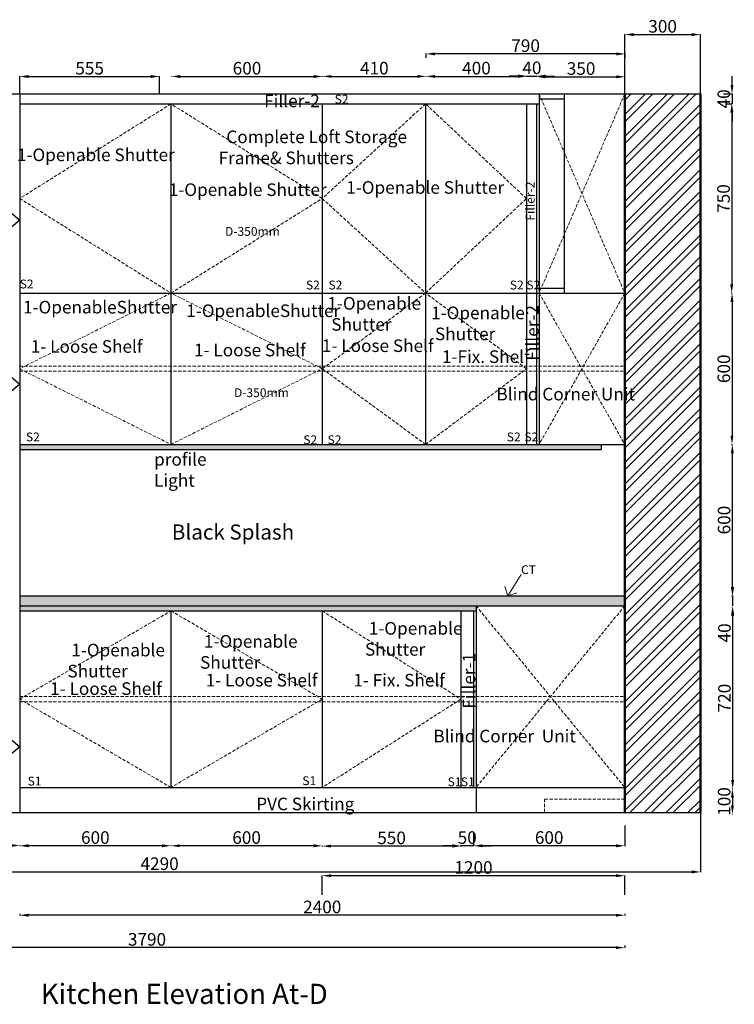
# Model space of a CAD drawing. Units: millimetres. Extents: x 407065 to 421840, y 1168257 to 1177792.
# Tile 14 of 17: x 415751 to 418585, y 1168277 to 1172181. Entities that reach past the tile are written whole.
import ezdxf

# ---------------------------------------------------------------- set-up
doc = ezdxf.new("R2010")
doc.units = ezdxf.units.MM
doc.linetypes.add('DASHED', pattern=[19.05, 12.7, -6.35])
for name, color, linetype, lineweight in [('A-ANNO-DIMS', 6, 'Continuous', 18), ('A-ANNO-SYMB', 6, 'Continuous', 18), ('A-ANNO-TEXT', 30, 'Continuous', 18), ('A-FURN', 3, 'Continuous', 25), ('A-FURN-HIDN', 7, 'DASHED', 18), ('A-FURN-PATT', 252, 'Continuous', 13), ('A-WALL', 7, 'Continuous', 50), ('A-WALL-PATT', 8, 'Continuous', 13)]:
    doc.layers.add(name, color=color, linetype=linetype, lineweight=lineweight)
doc.styles.get("Standard").update_dxf_attribs({"font": 'arial.ttf'})
doc.dimstyles.new('ISO-25', dxfattribs={"dimtxt": 50, "dimasz": 35, "dimexe": 1.25, "dimexo": 0.625, "dimtad": 1, "dimdec": 1, "dimtxsty": 'Standard', "dimcen": 35, "dimadec": 0, "dimazin": 0, "dimtfac": 1, "dimtdec": 1, "dimtmove": 0, "dimatfit": 3, "dimfxl": 1, "dimarcsym": 0})

# ---------------------------------------------------------------- blocks, each defined once
blk = doc.blocks.new('*D135')
at = {"layer": 'A-ANNO-DIMS', "color": 0, "lineweight": -2, "transparency": 16777216}
for p, q in [((415750.9, 1171887.4), (415750.9, 1171956.9)), ((415785.9, 1171955.6), (416270.9, 1171955.6)), ((416305.9, 1171887.4), (416305.9, 1171956.9))]:
    blk.add_line(p, q, dxfattribs=at)
at = {"layer": 'A-ANNO-DIMS', "color": 0, "transparency": 16777216}
for points in [[(415785.9, 1171961.5), (415785.9, 1171949.8), (415750.9, 1171955.6)], [(416270.9, 1171961.5), (416270.9, 1171949.8), (416305.9, 1171955.6)]]:
    blk.add_solid(points, dxfattribs=at)
at = {"layer": 'Defpoints', "color": 0, "transparency": 16777216}
for p in [(416305.9, 1171955.6), (415750.9, 1171886.8), (416305.9, 1171886.8)]:
    blk.add_point(p, dxfattribs=at)
at = {"layer": 'A-ANNO-DIMS', "color": 0, "transparency": 16777216, "insert": (416028.4, 1171981.7), "char_height": 50, "attachment_point": 5}
blk.add_mtext('555', dxfattribs=at)
blk = doc.blocks.new('*D136')
at = {"layer": 'A-ANNO-DIMS', "color": 0, "lineweight": -2, "transparency": 16777216}
for p, q in [((416352.5, 1171955.3), (416352.5, 1171954.4)), ((416387.5, 1171955.6), (416917.5, 1171955.6)), ((416952.5, 1171955.3), (416952.5, 1171954.4))]:
    blk.add_line(p, q, dxfattribs=at)
at = {"layer": 'A-ANNO-DIMS', "color": 0, "transparency": 16777216}
for points in [[(416387.5, 1171961.5), (416387.5, 1171949.8), (416352.5, 1171955.6)], [(416917.5, 1171961.5), (416917.5, 1171949.8), (416952.5, 1171955.6)]]:
    blk.add_solid(points, dxfattribs=at)
at = {"layer": 'Defpoints', "color": 0, "transparency": 16777216}
for p in [(416352.5, 1171955.9), (416952.5, 1171955.9), (416952.5, 1171955.6)]:
    blk.add_point(p, dxfattribs=at)
at = {"layer": 'A-ANNO-DIMS', "color": 0, "transparency": 16777216, "insert": (416652.5, 1171981.8), "char_height": 50, "attachment_point": 5}
blk.add_mtext('600', dxfattribs=at)
blk = doc.blocks.new('*D137')
at = {"layer": 'A-ANNO-DIMS', "color": 0, "lineweight": -2, "transparency": 16777216}
for p, q in [((416952.5, 1171955), (416952.5, 1171957.2)), ((416987.5, 1171955.9), (417327.5, 1171955.9)), ((417362.5, 1171955), (417362.5, 1171957.2))]:
    blk.add_line(p, q, dxfattribs=at)
at = {"layer": 'A-ANNO-DIMS', "color": 0, "transparency": 16777216}
for points in [[(416987.5, 1171961.7), (416987.5, 1171950.1), (416952.5, 1171955.9)], [(417327.5, 1171961.7), (417327.5, 1171950.1), (417362.5, 1171955.9)]]:
    blk.add_solid(points, dxfattribs=at)
at = {"layer": 'Defpoints', "color": 0, "transparency": 16777216}
for p in [(416952.5, 1171954.4), (417362.5, 1171955.9), (417362.5, 1171954.4)]:
    blk.add_point(p, dxfattribs=at)
at = {"layer": 'A-ANNO-DIMS', "color": 0, "transparency": 16777216, "insert": (417157.5, 1171982.1), "char_height": 50, "attachment_point": 5}
blk.add_mtext('410', dxfattribs=at)
blk = doc.blocks.new('*D138')
at = {"layer": 'A-ANNO-DIMS', "color": 0, "lineweight": -2, "transparency": 16777216}
for p, q in [((417362.5, 1171955), (417362.5, 1171957.3)), ((417397.5, 1171956.1), (417727.5, 1171956.1)), ((417762.5, 1171955), (417762.5, 1171957.3))]:
    blk.add_line(p, q, dxfattribs=at)
at = {"layer": 'A-ANNO-DIMS', "color": 0, "transparency": 16777216}
for points in [[(417397.5, 1171961.9), (417397.5, 1171950.2), (417362.5, 1171956.1)], [(417727.5, 1171961.9), (417727.5, 1171950.2), (417762.5, 1171956.1)]]:
    blk.add_solid(points, dxfattribs=at)
at = {"layer": 'Defpoints', "color": 0, "transparency": 16777216}
for p in [(417362.5, 1171954.4), (417762.5, 1171956.1), (417762.5, 1171954.4)]:
    blk.add_point(p, dxfattribs=at)
at = {"layer": 'A-ANNO-DIMS', "color": 0, "transparency": 16777216, "insert": (417562.5, 1171982.2), "char_height": 50, "attachment_point": 5}
blk.add_mtext('400', dxfattribs=at)
blk = doc.blocks.new('*D139')
at = {"layer": 'A-ANNO-DIMS', "color": 0, "lineweight": -2, "transparency": 16777216}
for p, q in [((417727.5, 1171957.3), (417692.5, 1171957.3)), ((417762.5, 1171955), (417762.5, 1171958.6)), ((417762.5, 1171957.3), (417802.5, 1171957.3)), ((417802.5, 1171955), (417802.5, 1171958.6)), ((417837.5, 1171957.3), (417872.5, 1171957.3))]:
    blk.add_line(p, q, dxfattribs=at)
at = {"layer": 'A-ANNO-DIMS', "color": 0, "transparency": 16777216}
for points in [[(417727.5, 1171963.2), (417727.5, 1171951.5), (417762.5, 1171957.3)], [(417837.5, 1171963.2), (417837.5, 1171951.5), (417802.5, 1171957.3)]]:
    blk.add_solid(points, dxfattribs=at)
at = {"layer": 'Defpoints', "color": 0, "transparency": 16777216}
for p in [(417762.5, 1171954.4), (417802.5, 1171957.3), (417802.5, 1171954.4)]:
    blk.add_point(p, dxfattribs=at)
at = {"layer": 'A-ANNO-DIMS', "color": 0, "transparency": 16777216, "insert": (417782.5, 1171983.5), "char_height": 50, "attachment_point": 5}
blk.add_mtext('40', dxfattribs=at)
blk = doc.blocks.new('*D140')
at = {"layer": 'A-ANNO-DIMS', "color": 0, "lineweight": -2, "transparency": 16777216}
for p, q in [((417802.5, 1171955), (417802.5, 1171955.6)), ((417837.5, 1171954.4), (418117.5, 1171954.4)), ((418152.5, 1171955), (418152.5, 1171955.6))]:
    blk.add_line(p, q, dxfattribs=at)
at = {"layer": 'A-ANNO-DIMS', "color": 0, "transparency": 16777216}
for points in [[(417837.5, 1171960.2), (417837.5, 1171948.5), (417802.5, 1171954.4)], [(418117.5, 1171960.2), (418117.5, 1171948.5), (418152.5, 1171954.4)]]:
    blk.add_solid(points, dxfattribs=at)
at = {"layer": 'Defpoints', "color": 0, "transparency": 16777216}
for p in [(417802.5, 1171954.4), (418152.5, 1171954.4), (418152.5, 1171954.4)]:
    blk.add_point(p, dxfattribs=at)
at = {"layer": 'A-ANNO-DIMS', "color": 0, "transparency": 16777216, "insert": (417977.5, 1171980.6), "char_height": 50, "attachment_point": 5}
blk.add_mtext('350', dxfattribs=at)
blk = doc.blocks.new('*D141')
at = {"layer": 'A-ANNO-DIMS', "color": 0, "lineweight": -2, "transparency": 16777216}
for p, q in [((417362.5, 1172030), (417362.5, 1172046.4)), ((418117.5, 1172045.1), (417397.5, 1172045.1)), ((418152.5, 1172030), (418152.5, 1172046.4))]:
    blk.add_line(p, q, dxfattribs=at)
at = {"layer": 'A-ANNO-DIMS', "color": 0, "transparency": 16777216}
for points in [[(417397.5, 1172050.9), (417397.5, 1172039.3), (417362.5, 1172045.1)], [(418117.5, 1172050.9), (418117.5, 1172039.3), (418152.5, 1172045.1)]]:
    blk.add_solid(points, dxfattribs=at)
at = {"layer": 'Defpoints', "color": 0, "transparency": 16777216}
for p in [(417362.5, 1172045.1), (417362.5, 1172029.4), (418152.5, 1172029.4)]:
    blk.add_point(p, dxfattribs=at)
at = {"layer": 'A-ANNO-DIMS', "color": 0, "transparency": 16777216, "insert": (417757.5, 1172071.3), "char_height": 50, "attachment_point": 5}
blk.add_mtext('790', dxfattribs=at)
blk = doc.blocks.new('*D142')
at = {"layer": 'A-ANNO-DIMS', "color": 0, "lineweight": -2, "transparency": 16777216}
for p, q in [((418576.1, 1171921.8), (418576.1, 1171956.8)), ((418542.5, 1171886.8), (418577.4, 1171886.8)), ((418576.1, 1171886.8), (418576.1, 1171846.8)), ((418551.7, 1171846.8), (418577.4, 1171846.8)), ((418576.1, 1171811.8), (418576.1, 1171776.8))]:
    blk.add_line(p, q, dxfattribs=at)
at = {"layer": 'A-ANNO-DIMS', "color": 0, "transparency": 16777216}
for points in [[(418570.3, 1171921.8), (418581.9, 1171921.8), (418576.1, 1171886.8)], [(418570.3, 1171811.8), (418581.9, 1171811.8), (418576.1, 1171846.8)]]:
    blk.add_solid(points, dxfattribs=at)
at = {"layer": 'Defpoints', "color": 0, "transparency": 16777216}
for p in [(418541.8, 1171886.8), (418551, 1171846.8), (418576.1, 1171846.8)]:
    blk.add_point(p, dxfattribs=at)
at = {"layer": 'A-ANNO-DIMS', "color": 0, "transparency": 16777216, "insert": (418550, 1171866.8), "char_height": 50, "attachment_point": 5, "rotation": 90}
blk.add_mtext('40', dxfattribs=at)
blk = doc.blocks.new('*D143')
at = {"layer": 'A-ANNO-DIMS', "color": 0, "lineweight": -2, "transparency": 16777216}
for p, q in [((418575.5, 1171846.8), (418573.7, 1171846.8)), ((418574.9, 1171811.8), (418574.9, 1171131.8)), ((418575.5, 1171096.8), (418573.7, 1171096.8))]:
    blk.add_line(p, q, dxfattribs=at)
at = {"layer": 'A-ANNO-DIMS', "color": 0, "transparency": 16777216}
for points in [[(418569.1, 1171811.8), (418580.7, 1171811.8), (418574.9, 1171846.8)], [(418569.1, 1171131.8), (418580.7, 1171131.8), (418574.9, 1171096.8)]]:
    blk.add_solid(points, dxfattribs=at)
at = {"layer": 'Defpoints', "color": 0, "transparency": 16777216}
for p in [(418576.1, 1171846.8), (418574.9, 1171096.8), (418576.1, 1171096.8)]:
    blk.add_point(p, dxfattribs=at)
at = {"layer": 'A-ANNO-DIMS', "color": 0, "transparency": 16777216, "insert": (418548.8, 1171471.8), "char_height": 50, "attachment_point": 5, "rotation": 90}
blk.add_mtext('750', dxfattribs=at)
blk = doc.blocks.new('*D144')
at = {"layer": 'A-ANNO-DIMS', "color": 0, "lineweight": -2, "transparency": 16777216}
for p, q in [((418574.3, 1171096.8), (418577.4, 1171096.8)), ((418576.1, 1171061.8), (418576.1, 1170531.8)), ((418574.3, 1170496.8), (418577.4, 1170496.8))]:
    blk.add_line(p, q, dxfattribs=at)
at = {"layer": 'A-ANNO-DIMS', "color": 0, "transparency": 16777216}
for points in [[(418570.3, 1171061.8), (418581.9, 1171061.8), (418576.1, 1171096.8)], [(418570.3, 1170531.8), (418581.9, 1170531.8), (418576.1, 1170496.8)]]:
    blk.add_solid(points, dxfattribs=at)
at = {"layer": 'Defpoints', "color": 0, "transparency": 16777216}
for p in [(418573.7, 1171096.8), (418573.7, 1170496.8), (418576.1, 1170496.8)]:
    blk.add_point(p, dxfattribs=at)
at = {"layer": 'A-ANNO-DIMS', "color": 0, "transparency": 16777216, "insert": (418550, 1170796.8), "char_height": 50, "attachment_point": 5, "rotation": 90}
blk.add_mtext('600', dxfattribs=at)
blk = doc.blocks.new('*D145')
at = {"layer": 'A-ANNO-DIMS', "color": 0, "lineweight": -2, "transparency": 16777216}
for p, q in [((418574.3, 1170496.8), (418578.6, 1170496.8)), ((418577.4, 1170461.8), (418577.4, 1169931.8)), ((418574.3, 1169896.8), (418578.6, 1169896.8))]:
    blk.add_line(p, q, dxfattribs=at)
at = {"layer": 'A-ANNO-DIMS', "color": 0, "transparency": 16777216}
for points in [[(418571.5, 1170461.8), (418583.2, 1170461.8), (418577.4, 1170496.8)], [(418571.5, 1169931.8), (418583.2, 1169931.8), (418577.4, 1169896.8)]]:
    blk.add_solid(points, dxfattribs=at)
at = {"layer": 'Defpoints', "color": 0, "transparency": 16777216}
for p in [(418573.7, 1170496.8), (418573.7, 1169896.8), (418577.4, 1169896.8)]:
    blk.add_point(p, dxfattribs=at)
at = {"layer": 'A-ANNO-DIMS', "color": 0, "transparency": 16777216, "insert": (418551.2, 1170196.8), "char_height": 50, "attachment_point": 5, "rotation": 90}
blk.add_mtext('600', dxfattribs=at)
blk = doc.blocks.new('*D146')
at = {"layer": 'A-ANNO-DIMS', "color": 0, "lineweight": -2, "transparency": 16777216}
for p, q in [((418578.6, 1169931.8), (418578.6, 1169966.8)), ((418578.6, 1169896.8), (418578.6, 1169856.8)), ((418579.2, 1169896.8), (418579.9, 1169896.8)), ((418579.2, 1169856.8), (418579.9, 1169856.8)), ((418578.6, 1169821.8), (418578.6, 1169712.1))]:
    blk.add_line(p, q, dxfattribs=at)
at = {"layer": 'A-ANNO-DIMS', "color": 0, "transparency": 16777216}
for points in [[(418572.8, 1169931.8), (418584.4, 1169931.8), (418578.6, 1169896.8)], [(418572.8, 1169821.8), (418584.4, 1169821.8), (418578.6, 1169856.8)]]:
    blk.add_solid(points, dxfattribs=at)
at = {"layer": 'Defpoints', "color": 0, "transparency": 16777216}
for p in [(418578.6, 1169896.8), (418578.6, 1169856.8), (418578.6, 1169856.8)]:
    blk.add_point(p, dxfattribs=at)
at = {"layer": 'A-ANNO-DIMS', "color": 0, "transparency": 16777216, "insert": (418552.5, 1169749.5), "char_height": 50, "attachment_point": 5, "rotation": 90}
blk.add_mtext('40', dxfattribs=at)
blk = doc.blocks.new('*D147')
at = {"layer": 'A-ANNO-DIMS', "color": 0, "lineweight": -2, "transparency": 16777216}
for p, q in [((418579.2, 1169851.1), (418579.9, 1169851.1)), ((418578.6, 1169816.1), (418578.6, 1169166.1)), ((418579.2, 1169131.1), (418579.9, 1169131.1))]:
    blk.add_line(p, q, dxfattribs=at)
at = {"layer": 'A-ANNO-DIMS', "color": 0, "transparency": 16777216}
for points in [[(418572.8, 1169816.1), (418584.4, 1169816.1), (418578.6, 1169851.1)], [(418572.8, 1169166.1), (418584.4, 1169166.1), (418578.6, 1169131.1)]]:
    blk.add_solid(points, dxfattribs=at)
at = {"layer": 'Defpoints', "color": 0, "transparency": 16777216}
for p in [(418578.6, 1169851.1), (418578.6, 1169131.1), (418578.6, 1169131.1)]:
    blk.add_point(p, dxfattribs=at)
at = {"layer": 'A-ANNO-DIMS', "color": 0, "transparency": 16777216, "insert": (418552.5, 1169491.1), "char_height": 50, "attachment_point": 5, "rotation": 90}
blk.add_mtext('720', dxfattribs=at)
blk = doc.blocks.new('*D148')
at = {"layer": 'A-ANNO-DIMS', "color": 0, "lineweight": -2, "transparency": 16777216}
for p, q in [((418578, 1169131.1), (418576.4, 1169131.1)), ((418577.7, 1169096.1), (418577.7, 1169066.1)), ((418578, 1169031.1), (418576.4, 1169031.1))]:
    blk.add_line(p, q, dxfattribs=at)
at = {"layer": 'A-ANNO-DIMS', "color": 0, "transparency": 16777216}
for points in [[(418571.8, 1169096.1), (418583.5, 1169096.1), (418577.7, 1169131.1)], [(418571.8, 1169066.1), (418583.5, 1169066.1), (418577.7, 1169031.1)]]:
    blk.add_solid(points, dxfattribs=at)
at = {"layer": 'Defpoints', "color": 0, "transparency": 16777216}
for p in [(418578.6, 1169131.1), (418577.7, 1169031.1), (418578.6, 1169031.1)]:
    blk.add_point(p, dxfattribs=at)
at = {"layer": 'A-ANNO-DIMS', "color": 0, "transparency": 16777216, "insert": (418551.5, 1169081.1), "char_height": 50, "attachment_point": 5, "rotation": 90}
blk.add_mtext('100', dxfattribs=at)
blk = doc.blocks.new('*D149')
at = {"layer": 'A-ANNO-DIMS', "color": 0, "lineweight": -2, "transparency": 16777216}
for p, q in [((418150.9, 1168985.5), (418150.9, 1168904.2)), ((417550.9, 1168959.3), (417550.9, 1168904.2)), ((418115.9, 1168905.4), (417585.9, 1168905.4))]:
    blk.add_line(p, q, dxfattribs=at)
at = {"layer": 'A-ANNO-DIMS', "color": 0, "transparency": 16777216}
for points in [[(417585.9, 1168911.3), (417585.9, 1168899.6), (417550.9, 1168905.4)], [(418115.9, 1168911.3), (418115.9, 1168899.6), (418150.9, 1168905.4)]]:
    blk.add_solid(points, dxfattribs=at)
at = {"layer": 'Defpoints', "color": 0, "transparency": 16777216}
for p in [(418150.9, 1168986.2), (417550.9, 1168959.9), (417550.9, 1168905.4)]:
    blk.add_point(p, dxfattribs=at)
at = {"layer": 'A-ANNO-DIMS', "color": 0, "transparency": 16777216, "insert": (417850.9, 1168931.6), "char_height": 50, "attachment_point": 5}
blk.add_mtext('600', dxfattribs=at)
blk = doc.blocks.new('*D150')
at = {"layer": 'A-ANNO-DIMS', "color": 0, "lineweight": -2, "transparency": 16777216}
for p, q in [((417465.9, 1168905.4), (417430.9, 1168905.4)), ((417500.9, 1168904.8), (417500.9, 1168906.7)), ((417550.9, 1168905.4), (417500.9, 1168905.4)), ((417550.9, 1168904.8), (417550.9, 1168906.7)), ((417585.9, 1168905.4), (417620.9, 1168905.4))]:
    blk.add_line(p, q, dxfattribs=at)
at = {"layer": 'A-ANNO-DIMS', "color": 0, "transparency": 16777216}
for points in [[(417465.9, 1168911.3), (417465.9, 1168899.6), (417500.9, 1168905.4)], [(417585.9, 1168911.3), (417585.9, 1168899.6), (417550.9, 1168905.4)]]:
    blk.add_solid(points, dxfattribs=at)
at = {"layer": 'Defpoints', "color": 0, "transparency": 16777216}
for p in [(417500.9, 1168905.4), (417500.9, 1168904.2), (417550.9, 1168904.2)]:
    blk.add_point(p, dxfattribs=at)
at = {"layer": 'A-ANNO-DIMS', "color": 0, "transparency": 16777216, "insert": (417525.9, 1168931.6), "char_height": 50, "attachment_point": 5}
blk.add_mtext('50', dxfattribs=at)
blk = doc.blocks.new('*D151')
at = {"layer": 'A-ANNO-DIMS', "color": 0, "lineweight": -2, "transparency": 16777216}
for p, q in [((416950.9, 1168904.8), (416950.9, 1168902.9)), ((417465.9, 1168904.2), (416985.9, 1168904.2)), ((417500.9, 1168904.8), (417500.9, 1168902.9))]:
    blk.add_line(p, q, dxfattribs=at)
at = {"layer": 'A-ANNO-DIMS', "color": 0, "transparency": 16777216}
for points in [[(416985.9, 1168910), (416985.9, 1168898.4), (416950.9, 1168904.2)], [(417465.9, 1168910), (417465.9, 1168898.4), (417500.9, 1168904.2)]]:
    blk.add_solid(points, dxfattribs=at)
at = {"layer": 'Defpoints', "color": 0, "transparency": 16777216}
for p in [(416950.9, 1168905.4), (416950.9, 1168904.2), (417500.9, 1168905.4)]:
    blk.add_point(p, dxfattribs=at)
at = {"layer": 'A-ANNO-DIMS', "color": 0, "transparency": 16777216, "insert": (417225.9, 1168930.3), "char_height": 50, "attachment_point": 5}
blk.add_mtext('550', dxfattribs=at)
blk = doc.blocks.new('*D152')
at = {"layer": 'A-ANNO-DIMS', "color": 0, "lineweight": -2, "transparency": 16777216}
for p, q in [((416350.9, 1168906.1), (416350.9, 1168906.7)), ((416915.9, 1168905.4), (416385.9, 1168905.4)), ((416950.9, 1168906.1), (416950.9, 1168906.7))]:
    blk.add_line(p, q, dxfattribs=at)
at = {"layer": 'A-ANNO-DIMS', "color": 0, "transparency": 16777216}
for points in [[(416385.9, 1168911.3), (416385.9, 1168899.6), (416350.9, 1168905.4)], [(416915.9, 1168911.3), (416915.9, 1168899.6), (416950.9, 1168905.4)]]:
    blk.add_solid(points, dxfattribs=at)
at = {"layer": 'Defpoints', "color": 0, "transparency": 16777216}
for p in [(416350.9, 1168905.4), (416350.9, 1168905.4), (416950.9, 1168905.4)]:
    blk.add_point(p, dxfattribs=at)
at = {"layer": 'A-ANNO-DIMS', "color": 0, "transparency": 16777216, "insert": (416650.9, 1168931.6), "char_height": 50, "attachment_point": 5}
blk.add_mtext('600', dxfattribs=at)
blk = doc.blocks.new('*D153')
at = {"layer": 'A-ANNO-DIMS', "color": 0, "lineweight": -2, "transparency": 16777216}
for p, q in [((415750.9, 1168906.1), (415750.9, 1168904.2)), ((416315.9, 1168905.4), (415785.9, 1168905.4)), ((416350.9, 1168906.1), (416350.9, 1168904.2))]:
    blk.add_line(p, q, dxfattribs=at)
at = {"layer": 'A-ANNO-DIMS', "color": 0, "transparency": 16777216}
for points in [[(415785.9, 1168911.3), (415785.9, 1168899.6), (415750.9, 1168905.4)], [(416315.9, 1168911.3), (416315.9, 1168899.6), (416350.9, 1168905.4)]]:
    blk.add_solid(points, dxfattribs=at)
at = {"layer": 'Defpoints', "color": 0, "transparency": 16777216}
for p in [(415750.9, 1168906.7), (415750.9, 1168905.4), (416350.9, 1168906.7)]:
    blk.add_point(p, dxfattribs=at)
at = {"layer": 'A-ANNO-DIMS', "color": 0, "transparency": 16777216, "insert": (416050.9, 1168931.6), "char_height": 50, "attachment_point": 5}
blk.add_mtext('600', dxfattribs=at)
blk = doc.blocks.new('*D154')
at = {"layer": 'A-ANNO-DIMS', "color": 0, "lineweight": -2, "transparency": 16777216}
for p, q in [((415480.9, 1168907.3), (415480.9, 1168907.9)), ((415715.9, 1168906.7), (415515.9, 1168906.7)), ((415750.9, 1168907.3), (415750.9, 1168907.9))]:
    blk.add_line(p, q, dxfattribs=at)
at = {"layer": 'A-ANNO-DIMS', "color": 0, "transparency": 16777216}
for points in [[(415515.9, 1168912.5), (415515.9, 1168900.9), (415480.9, 1168906.7)], [(415715.9, 1168912.5), (415715.9, 1168900.9), (415750.9, 1168906.7)]]:
    blk.add_solid(points, dxfattribs=at)
at = {"layer": 'Defpoints', "color": 0, "transparency": 16777216}
for p in [(415480.9, 1168906.7), (415480.9, 1168906.7), (415750.9, 1168906.7)]:
    blk.add_point(p, dxfattribs=at)
at = {"layer": 'A-ANNO-DIMS', "color": 0, "transparency": 16777216, "insert": (415615.9, 1168932.8), "char_height": 50, "attachment_point": 5}
blk.add_mtext('270', dxfattribs=at)
blk = doc.blocks.new('*D156')
at = {"layer": 'A-ANNO-DIMS', "color": 0, "lineweight": -2, "transparency": 16777216}
for p, q in [((416950.9, 1168710.6), (416950.9, 1168788.2)), ((418115.9, 1168786.9), (416985.9, 1168786.9)), ((418150.9, 1168710.6), (418150.9, 1168788.2))]:
    blk.add_line(p, q, dxfattribs=at)
at = {"layer": 'A-ANNO-DIMS', "color": 0, "transparency": 16777216}
for points in [[(416985.9, 1168792.8), (416985.9, 1168781.1), (416950.9, 1168786.9)], [(418115.9, 1168792.8), (418115.9, 1168781.1), (418150.9, 1168786.9)]]:
    blk.add_solid(points, dxfattribs=at)
at = {"layer": 'Defpoints', "color": 0, "transparency": 16777216}
for p in [(416950.9, 1168786.9), (416950.9, 1168709.9), (418150.9, 1168709.9)]:
    blk.add_point(p, dxfattribs=at)
at = {"layer": 'A-ANNO-DIMS', "color": 0, "transparency": 16777216, "insert": (417550.9, 1168813.1), "char_height": 50, "attachment_point": 5}
blk.add_mtext('1200', dxfattribs=at)
blk = doc.blocks.new('*D157')
at = {"layer": 'A-ANNO-DIMS', "color": 0, "lineweight": -2, "transparency": 16777216}
for p, q in [((415750.9, 1168635.3), (415750.9, 1168629)), ((418115.9, 1168630.2), (415785.9, 1168630.2)), ((418150.9, 1168635.3), (418150.9, 1168629))]:
    blk.add_line(p, q, dxfattribs=at)
at = {"layer": 'A-ANNO-DIMS', "color": 0, "transparency": 16777216}
for points in [[(415785.9, 1168636), (415785.9, 1168624.4), (415750.9, 1168630.2)], [(418115.9, 1168636), (418115.9, 1168624.4), (418150.9, 1168630.2)]]:
    blk.add_solid(points, dxfattribs=at)
at = {"layer": 'Defpoints', "color": 0, "transparency": 16777216}
for p in [(415750.9, 1168635.9), (415750.9, 1168630.2), (418150.9, 1168635.9)]:
    blk.add_point(p, dxfattribs=at)
at = {"layer": 'A-ANNO-DIMS', "color": 0, "transparency": 16777216, "insert": (416950.9, 1168656.4), "char_height": 50, "attachment_point": 5}
blk.add_mtext('2400', dxfattribs=at)
blk = doc.blocks.new('*D158')
at = {"layer": 'A-ANNO-DIMS', "color": 0, "lineweight": -2, "transparency": 16777216}
for p, q in [((414360.9, 1168509.6), (414360.9, 1168500.5)), ((418115.9, 1168501.7), (414395.9, 1168501.7)), ((418150.9, 1168509.6), (418150.9, 1168500.5))]:
    blk.add_line(p, q, dxfattribs=at)
at = {"layer": 'A-ANNO-DIMS', "color": 0, "transparency": 16777216}
for points in [[(414395.9, 1168507.5), (414395.9, 1168495.9), (414360.9, 1168501.7)], [(418115.9, 1168507.5), (418115.9, 1168495.9), (418150.9, 1168501.7)]]:
    blk.add_solid(points, dxfattribs=at)
at = {"layer": 'Defpoints', "color": 0, "transparency": 16777216}
for p in [(414360.9, 1168510.3), (414360.9, 1168501.7), (418150.9, 1168510.3)]:
    blk.add_point(p, dxfattribs=at)
at = {"layer": 'A-ANNO-DIMS', "color": 0, "transparency": 16777216, "insert": (416255.9, 1168527.9), "char_height": 50, "attachment_point": 5}
blk.add_mtext('3790', dxfattribs=at)
blk = doc.blocks.new('*D219')
at = {"layer": 'A-ANNO-DIMS', "color": 0, "lineweight": -2, "transparency": 16777216}
for p, q in [((414160.9, 1169036.2), (414160.9, 1168800.6)), ((418450.9, 1169036.2), (418450.9, 1168800.6)), ((414195.9, 1168801.8), (418415.9, 1168801.8))]:
    blk.add_line(p, q, dxfattribs=at)
at = {"layer": 'A-ANNO-DIMS', "color": 0, "transparency": 16777216}
for points in [[(414195.9, 1168807.7), (414195.9, 1168796), (414160.9, 1168801.8)], [(418415.9, 1168807.7), (418415.9, 1168796), (418450.9, 1168801.8)]]:
    blk.add_solid(points, dxfattribs=at)
at = {"layer": 'Defpoints', "color": 0, "transparency": 16777216}
for p in [(414160.9, 1169036.8), (418450.9, 1169036.8), (418450.9, 1168801.8)]:
    blk.add_point(p, dxfattribs=at)
at = {"layer": 'A-ANNO-DIMS', "color": 0, "transparency": 16777216, "insert": (416305.9, 1168828), "char_height": 50, "attachment_point": 5}
blk.add_mtext('4290', dxfattribs=at)
blk = doc.blocks.new('*D221')
at = {"layer": 'A-ANNO-DIMS', "color": 0, "lineweight": -2, "transparency": 16777216}
for p, q in [((418150.9, 1171887.4), (418150.9, 1172123.1)), ((418185.9, 1172121.8), (418415.9, 1172121.8)), ((418450.9, 1171887.4), (418450.9, 1172123.1))]:
    blk.add_line(p, q, dxfattribs=at)
at = {"layer": 'A-ANNO-DIMS', "color": 0, "transparency": 16777216}
for points in [[(418185.9, 1172127.7), (418185.9, 1172116), (418150.9, 1172121.8)], [(418415.9, 1172127.7), (418415.9, 1172116), (418450.9, 1172121.8)]]:
    blk.add_solid(points, dxfattribs=at)
at = {"layer": 'Defpoints', "color": 0, "transparency": 16777216}
for p in [(418450.9, 1172121.8), (418150.9, 1171886.8), (418450.9, 1171886.8)]:
    blk.add_point(p, dxfattribs=at)
at = {"layer": 'A-ANNO-DIMS', "color": 0, "transparency": 16777216, "insert": (418300.9, 1172148), "char_height": 50, "attachment_point": 5}
blk.add_mtext('300', dxfattribs=at)

msp = doc.modelspace()

# ---------------------------------------------------------------- hatches: boundary and pattern name
at = {"layer": 'A-FURN-PATT'}
h = msp.add_hatch(color=256, dxfattribs=at)
h.dxf.hatch_style = 1
h.paths.add_polyline_path([(418057.1221, 1170496.8201), (415750.8552, 1170496.8201), (415750.8552, 1170476.8201), (418057.1221, 1170476.8201)])
h = msp.add_hatch(color=256, dxfattribs=at)
h.dxf.hatch_style = 1
h.paths.add_polyline_path([(418057.1221, 1170496.8201), (415750.8552, 1170496.8201), (415750.8552, 1170476.8201), (418057.1221, 1170476.8201)])
h = msp.add_hatch(dxfattribs=at)
h.set_pattern_fill('AR-CONC', color=256, scale=0.26, angle=180)
h.set_pattern_definition([(230, (-5401.863, -112.548), (-47.3680139, 4.1441622), [4.953, -54.483]), (175, (-5401.863, -112.55), (9.1632896, -49.6747798), [3.9624, -43.5865519]), (280.4514447, (-5405.81, -112.202), (-38.2047242, -45.5306155), [4.2094023, -46.3034636]), (226.1842, (-5401.863, -125.756), (-70.4805506, 10.9310053), [7.4295, -81.7245]), (276.6355576, (-5407.736, -124.845), (-61.725075, -64.3307924), [6.314106, -69.455258]), (171.184151, (-5401.86, -125.756), (-61.725075, -64.3307924), [5.9435914, -65.3795303]), (201, (-5408.467, -122.454), (-39.4197417, 26.5889515), [4.953, -54.483]), (146, (-5408.467, -122.454), (-16.0685274, -47.8888712), [3.9624, -43.5864]), (251.451445, (-5411.75, -120.24), (-55.488269, -21.2999199), [4.2094023, -46.3033838]), (217.5, (-5401.863, -112.548), (-0.80303685, -21.9843101), [0, -43.05808, 0, -44.2468, 0, -43.7515]), (187.5, (-5401.863, -112.548), (-17.37311225, -26.04694945), [0, -25.22728, 0, -42.06748, 0, -16.6751]), (147.5, (-5387.136, -112.548), (-35.25355474, 1.48947344), [0, -16.51, 0, -51.5112, 0, -68.3514]), (137.5, (-5380.532, -112.548), (-38.51358716, -6.6108877), [0, -21.463, 0, -34.20872, 0, -48.5394])])
h.paths.add_polyline_path([(418150.8552, 1169896.8201), (415750.8552, 1169896.8201), (415750.8552, 1169856.8201), (418150.8552, 1169856.8201)])
h = msp.add_hatch(color=256, dxfattribs=at)
h.dxf.hatch_style = 1
h.paths.add_polyline_path([(417560.8552, 1169856.8201), (415750.8552, 1169856.8201), (415750.8552, 1169836.8201), (417560.8552, 1169836.8201)])
at = {"layer": 'A-WALL-PATT'}
h = msp.add_hatch(dxfattribs=at)
h.set_pattern_fill('ANSI32', color=256, scale=6.4, angle=180)
h.set_pattern_definition([(225, (-18706.866, -112.55), (43.1052294, -43.1052294), []), (225, (-18735.6, -112.55), (43.1052294, -43.1052294), [])])
h.paths.add_polyline_path([(418450.8552, 1171886.8201), (418150.8552, 1171886.8201), (418150.8552, 1169036.8201), (418450.8552, 1169036.8201)])

# ---------------------------------------------------------------- linework, layer by layer
at = {"layer": 'A-ANNO-SYMB'}
for p, q in [((417739.2747, 1169981.5149), (417687.4807, 1169896.8201)), ((417687.4807, 1169896.8201), (417675.3481, 1169933.4457)), ((417687.4807, 1169896.8201), (417722.1222, 1169908.2954))]:
    msp.add_line(p, q, dxfattribs=at)
at = {"layer": 'A-FURN'}
for p, q in [((414160.8552, 1171886.8201), (418450.8552, 1171886.8201)), ((415750.8552, 1171886.8201), (415750.8552, 1169036.8201)), ((417810.8552, 1171886.8201), (417810.8552, 1170496.8201)), ((417810.8552, 1171866.8201), (417910.8552, 1171866.8201)), ((417910.8552, 1171886.8201), (417910.8552, 1171096.8201)), ((415750.8552, 1171846.8201), (417810.8552, 1171846.8201)), ((416350.8552, 1171846.8201), (416350.8552, 1170496.8201)), ((416950.8552, 1171846.8201), (416950.8552, 1170496.8201)), ((417360.8552, 1171846.8201), (417360.8552, 1170496.8201)), ((417760.8552, 1171846.8201), (417760.8552, 1170496.8201)), ((417800.8552, 1171846.8201), (417800.8552, 1170496.8201)), ((415750.8552, 1171096.8201), (418150.8552, 1171096.8201)), ((417800.8552, 1171116.8201), (417910.8552, 1171116.8201)), ((415750.8552, 1170496.8201), (418150.8552, 1170496.8201)), ((418057.1221, 1170496.8201), (418057.1221, 1170476.8201)), ((415750.8552, 1170476.8201), (418057.1221, 1170476.8201)), ((415750.8552, 1169896.8201), (418150.8552, 1169896.8201)), ((415750.8552, 1169856.8201), (418150.8552, 1169856.8201)), ((415750.8552, 1169836.8201), (417560.8552, 1169836.8201)), ((416350.8552, 1169836.8201), (416350.8552, 1169136.8201)), ((416950.8552, 1169836.8201), (416950.8552, 1169136.8201)), ((417500.8552, 1169836.8201), (417500.8552, 1169136.8201)), ((417550.8552, 1169836.8201), (417550.8552, 1169136.8201)), ((417560.8552, 1169856.8201), (417560.8552, 1169036.8201)), ((415750.8552, 1169136.8201), (418150.8552, 1169136.8201)), ((414160.8552, 1169036.8201), (418450.8552, 1169036.8201))]:
    msp.add_line(p, q, dxfattribs=at)
for points in [[(415692.9322, 1171434.2902), (415750.8552, 1171385.6064), (415692.9322, 1171336.9226)], [(415692.9322, 1170784.6991), (415750.8552, 1170736.0153), (415692.9322, 1170687.3315)], [(415692.9322, 1169346.8751), (415750.8552, 1169298.1913), (415692.9322, 1169249.5075)]]:
    msp.add_lwpolyline(points, close=True, dxfattribs=at)
at = {"layer": 'A-FURN-HIDN'}
for p, q in [((418150.8552, 1171886.8201), (417810.8552, 1171096.8201)), ((417810.8552, 1171886.8201), (418150.8552, 1171096.8201)), ((416350.8552, 1171846.8201), (415750.8552, 1171471.8201)), ((416950.8552, 1171471.8201), (416350.8552, 1171846.8201)), ((417360.8552, 1171846.8201), (416950.8552, 1171471.8201)), ((417760.8552, 1171471.8201), (417360.8552, 1171846.8201)), ((415750.8552, 1171471.8201), (416350.8552, 1171096.8201)), ((416350.8552, 1171096.8201), (416950.8552, 1171471.8201)), ((416950.8552, 1171471.8201), (417360.8552, 1171096.8201)), ((417360.8552, 1171096.8201), (417760.8552, 1171471.8201)), ((416350.8552, 1171096.8201), (415750.8552, 1170796.8201)), ((416950.8552, 1170796.8201), (416350.8552, 1171096.8201)), ((417360.8552, 1171096.8201), (416950.8552, 1170796.8201)), ((417760.8552, 1170796.8201), (417360.8552, 1171096.8201)), ((418150.8552, 1171096.8201), (417810.8552, 1170496.8201)), ((417810.8552, 1171096.8201), (418150.8552, 1170496.8201)), ((415750.8552, 1170806.8201), (418150.8552, 1170806.8201)), ((415750.8552, 1170796.8201), (416350.8552, 1170496.8201)), ((415750.8552, 1170786.8201), (418150.8552, 1170786.8201)), ((416350.8552, 1170496.8201), (416950.8552, 1170796.8201)), ((416950.8552, 1170796.8201), (417360.8552, 1170496.8201)), ((417360.8552, 1170496.8201), (417760.8552, 1170796.8201)), ((415750.8552, 1169486.8201), (416350.8552, 1169836.8201)), ((416350.8552, 1169836.8201), (416950.8552, 1169486.8201)), ((416950.8552, 1169836.8201), (417500.8552, 1169486.8201)), ((418150.8552, 1169856.8201), (417560.8552, 1169136.8201)), ((417560.8552, 1169856.8201), (418150.8552, 1169136.8201)), ((415750.8552, 1169496.8201), (418150.8552, 1169496.8201)), ((416350.8552, 1169136.8201), (415750.8552, 1169486.8201)), ((416950.8552, 1169486.8201), (416350.8552, 1169136.8201)), ((417500.8552, 1169486.8201), (416950.8552, 1169136.8201)), ((415750.8552, 1169476.8201), (418150.8552, 1169476.8201)), ((418150.8552, 1169090.7294), (417832.5253, 1169090.7294)), ((417832.5253, 1169090.7294), (417832.5253, 1169036.8201))]:
    msp.add_line(p, q, dxfattribs=at)
at = {"layer": 'A-WALL'}
for p, q in [((418150.8552, 1171886.8201), (418150.8552, 1169036.8201)), ((418450.8552, 1171886.8201), (418450.8552, 1169036.8201)), ((418150.8552, 1169090.7294), (418150.8552, 1169090.7294))]:
    msp.add_line(p, q, dxfattribs=at)

# ---------------------------------------------------------------- texts
at = {"layer": 'A-ANNO-TEXT', "attachment_point": 1}
for s, width, insert, char_height in [('     Filler-2', 382.409863, (416643.9283, 1171883.9509), 50), ('S2', 382.409863, (417000.1668, 1171883.0139), 35), ('  Complete Loft Storage     Frame& Shutters', 1053.70789, (416539.8395, 1171741.2731), 50), (' 1-Openable Shutter', 721.424123, (415724.6749, 1171670.0044), 50), (' 1-Openable Shutter', 721.424123, (416326.9461, 1171531.8081), 50), (' 1-Openable Shutter', 721.424123, (417030.7631, 1171540.5546), 50), ('  D-350mm', 382.409863, (416543.9892, 1171358.9274), 35), ('S2', 382.409863, (415750.8552, 1171150.3282), 35), ('S2', 382.409863, (416886.3271, 1171146.3208), 35), ('S2', 382.409863, (416975.6359, 1171146.3208), 35), ('S2', 382.409863, (417694.8634, 1171146.3208), 35), ('S2', 382.409863, (417760.8552, 1171146.3208), 35), ('     1-Openable\\P      Shutter', 520.083559, (416894.9585, 1171081.0373), 50), (' 1-OpenableShutter', 520.083559, (415764.101, 1171065.9506), 50), (' 1-OpenableShutter', 520.083559, (416411.4779, 1171051.7704), 50), ('     1-Openable\\P      Shutter', 520.083559, (417306.2999, 1171043.3448), 50), ('1- Loose Shelf', 477.976646, (415794.9207, 1170910.1409), 50), ('1- Loose Shelf', 477.976646, (416442.2976, 1170895.9608), 50), ('1- Loose Shelf', 477.976646, (416949.5829, 1170913.2769), 50), ('  1-Fix. Shelf', 448.437733, (417395.3103, 1170869.8427), 50), ('  D-350mm', 382.409863, (416579.5804, 1170719.3733), 35), ('Blind Corner Unit', 550.954957, (417641.7198, 1170721.4003), 50), ('S2', 382.409863, (415775.761, 1170543.9396), 35), ('S2', 382.409863, (416875.7419, 1170533.0139), 35), ('S2', 382.409863, (416971.9145, 1170533.0139), 35), ('S2', 382.409863, (417682.9245, 1170543.9396), 35), ('S2', 382.409863, (417752.9147, 1170543.9396), 35), ('profile Light', 382.409863, (416283.9624, 1170462.6281), 50), ('Black Splash', 506.516765, (416354.2446, 1170179.45), 60), ('CT', 382.409863, (417739.2747, 1170017.7087), 35), (' 1-Openable   Shutter', 520.083559, (417120.2948, 1169792.5362), 50), (' 1-Openable   Shutter', 520.083559, (416466.2693, 1169740.8409), 50), (' 1-Openable   Shutter', 520.083559, (415940.3071, 1169706.3804), 50), ('1- Loose Shelf', 494.500039, (415871.7347, 1169553.606), 50), ('1- Loose Shelf', 504.846908, (416488.7511, 1169587.014), 50), ('1- Fix. Shelf', 382.409863, (417074.2638, 1169587.014), 50), ('Blind Corner  Unit', 949.759098, (417391.7198, 1169365.4765), 50), ('S1', 382.409863, (415782.2456, 1169179.5391), 35), ('S1', 382.409863, (416871.7755, 1169180.9456), 35), ('S1', 382.409863, (417448.1482, 1169176.8149), 35), ('S1', 382.409863, (417500.8552, 1169176.8149), 35), ('    PVC Skirting', 572.580594, (416627.8044, 1169096.2775), 50), ('Kitchen Elevation At-D', 1357.183536, (415834.8076, 1168358.3661), 80)]:
    msp.add_mtext_dynamic_manual_height_columns(s, width=width, gutter_width=12.5, heights=[0], dxfattribs=dict(at, insert=insert, char_height=char_height))
at = {"layer": 'A-ANNO-TEXT', "attachment_point": 1, "rotation": 90}
for s, insert, char_height in [('     Filler-2', (417758.3544, 1171330.6021), 35), ('     Filler-2', (417759.5904, 1170751.886), 50), ('     Filler-1', (417508.1416, 1169372.8188), 50)]:
    msp.add_mtext_dynamic_manual_height_columns(s, width=382.409863, gutter_width=12.5, heights=[0], dxfattribs=dict(at, insert=insert, char_height=char_height))

# ---------------------------------------------------------------- dimensions: what is measured, and where the dimension line sits
at = {"layer": 'A-ANNO-DIMS'}
for base, p1, p2, override, picture, middle in [((418450.8552, 1172121.8201), (418150.8552, 1171886.8201), (418450.8552, 1171886.8201), {"dimdec": 0, "dimlfac": 1, "dimrnd": 0, "dimzin": 0, "dimdsep": 46, "dimlunit": 2}, '*D221', (418300.8552, 1172147.9908)), ((417362.5195, 1172045.1024), (418152.5195, 1172029.3713), (417362.5195, 1172029.3713), {"dimclrd": 0, "dimclre": 0, "dimclrt": 0}, '*D141', (417757.5195, 1172071.2561)), ((417762.5195, 1171956.0813), (417362.5195, 1171954.3801), (417762.5195, 1171954.3801), {"dimclrd": 0, "dimclre": 0, "dimclrt": 0}, '*D138', (417562.5195, 1171982.235)), ((416305.8552, 1171955.6301), (415750.8552, 1171886.8201), (416305.8552, 1171886.8201), {"dimclrd": 0, "dimclre": 0, "dimclrt": 0}, '*D135', (416028.3552, 1171981.6815)), ((416952.5195, 1171955.6301), (416352.5195, 1171955.9075), (416952.5195, 1171955.9075), {"dimclrd": 0, "dimclre": 0, "dimclrt": 0}, '*D136', (416652.5195, 1171981.7838)), ((417362.5195, 1171955.9075), (416952.5195, 1171954.3801), (417362.5195, 1171954.3801), {"dimclrd": 0, "dimclre": 0, "dimclrt": 0}, '*D137', (417157.5195, 1171982.0612)), ((418152.5195, 1171954.3801), (417802.5195, 1171954.3801), (418152.5195, 1171954.3801), {"dimclrd": 0, "dimclre": 0, "dimclrt": 0}, '*D140', (417977.5195, 1171980.5508)), ((418450.8552, 1168801.8201), (414160.8552, 1169036.8201), (418450.8552, 1169036.8201), {"dimdec": 0, "dimlfac": 1, "dimrnd": 0, "dimzin": 0, "dimdsep": 46, "dimlunit": 2}, '*D219', (416305.8552, 1168827.9738)), ((417550.8552, 1168905.4429), (418150.8552, 1168986.1655), (417550.8552, 1168959.9482), {"dimclrd": 0, "dimclre": 0, "dimclrt": 0}, '*D149', (417850.8552, 1168931.5966)), ((415480.8552, 1168906.6929), (415750.8552, 1168906.6929), (415480.8552, 1168906.6929), {"dimclrd": 0, "dimclre": 0, "dimclrt": 0}, '*D154', (415615.8552, 1168932.8466)), ((415750.8552, 1168905.4429), (416350.8552, 1168906.6929), (415750.8552, 1168906.6929), {"dimclrd": 0, "dimclre": 0, "dimclrt": 0}, '*D153', (416050.8552, 1168931.5966)), ((416350.8552, 1168905.4429), (416950.8552, 1168905.4429), (416350.8552, 1168905.4429), {"dimclrd": 0, "dimclre": 0, "dimclrt": 0}, '*D152', (416650.8552, 1168931.5966)), ((416950.8552, 1168904.1929), (417500.8552, 1168905.4429), (416950.8552, 1168905.4429), {"dimclrd": 0, "dimclre": 0, "dimclrt": 0}, '*D151', (417225.8552, 1168930.3466)), ((416950.8552, 1168786.9182), (418150.8552, 1168709.9321), (416950.8552, 1168709.9321), {"dimclrd": 0, "dimclre": 0, "dimclrt": 0}, '*D156', (417550.8552, 1168813.0719)), ((415750.8552, 1168630.2148), (418150.8552, 1168635.887), (415750.8552, 1168635.887), {"dimclrd": 0, "dimclre": 0, "dimclrt": 0}, '*D157', (416950.8552, 1168656.3685)), ((414360.8552, 1168501.7014), (418150.8552, 1168510.2523), (414360.8552, 1168510.2523), {"dimclrd": 0, "dimclre": 0, "dimclrt": 0}, '*D158', (416255.8552, 1168527.8721))]:
    dim = msp.add_linear_dim(base=base, p1=p1, p2=p2, dimstyle='ISO-25', override=override, dxfattribs=at)
    dim.commit()
    dim.dimension.update_dxf_attribs({"geometry": picture, "text_midpoint": middle})
for base, p1, p2, picture, middle in [((417802.5195, 1171957.3313), (417762.5195, 1171954.3801), (417802.5195, 1171954.3801), '*D139', (417782.5195, 1171957.3313)), ((417500.8552, 1168905.4429), (417550.8552, 1168904.1929), (417500.8552, 1168904.1929), '*D150', (417525.8552, 1168905.4429))]:
    dim = msp.add_linear_dim(base=base, p1=p1, p2=p2, dimstyle='ISO-25', override={"dimclrd": 0, "dimclre": 0, "dimclrt": 0}, dxfattribs=at)
    dim.commit()
    dim.dimension.update_dxf_attribs({"geometry": picture, "text_midpoint": middle, "dimtype": 160})
for base, p1, p2, picture, middle in [((418576.1098, 1171846.8201), (418541.8392, 1171886.8201), (418551.0491, 1171846.8201), '*D142', (418576.1098, 1171866.8201)), ((418577.6723, 1169031.12), (418578.6098, 1169131.12), (418578.6098, 1169031.12), '*D148', (418577.6723, 1169081.12))]:
    dim = msp.add_linear_dim(base=base, p1=p1, p2=p2, angle=90, dimstyle='ISO-25', override={"dimclrd": 0, "dimclre": 0, "dimclrt": 0}, dxfattribs=at)
    dim.commit()
    dim.dimension.update_dxf_attribs({"geometry": picture, "text_midpoint": middle, "dimtype": 160})
for base, p1, p2, picture, middle in [((418574.9118, 1171096.8201), (418576.1098, 1171846.8201), (418576.1098, 1171096.8201), '*D143', (418548.7581, 1171471.8201)), ((418576.1098, 1170496.8201), (418573.6618, 1171096.8201), (418573.6618, 1170496.8201), '*D144', (418549.9561, 1170796.8201)), ((418577.3598, 1169896.8201), (418573.6618, 1170496.8201), (418573.6618, 1169896.8201), '*D145', (418551.2061, 1170196.8201)), ((418578.6098, 1169856.8201), (418578.6098, 1169896.8201), (418578.6098, 1169856.8201), '*D146', (418552.4561, 1169749.4625)), ((418578.6098, 1169131.12), (418578.6098, 1169851.12), (418578.6098, 1169131.12), '*D147', (418552.4561, 1169491.12))]:
    dim = msp.add_linear_dim(base=base, p1=p1, p2=p2, angle=90, dimstyle='ISO-25', override={"dimclrd": 0, "dimclre": 0, "dimclrt": 0}, dxfattribs=at)
    dim.commit()
    dim.dimension.update_dxf_attribs({"geometry": picture, "text_midpoint": middle})

doc.saveas('drawing.dxf')
